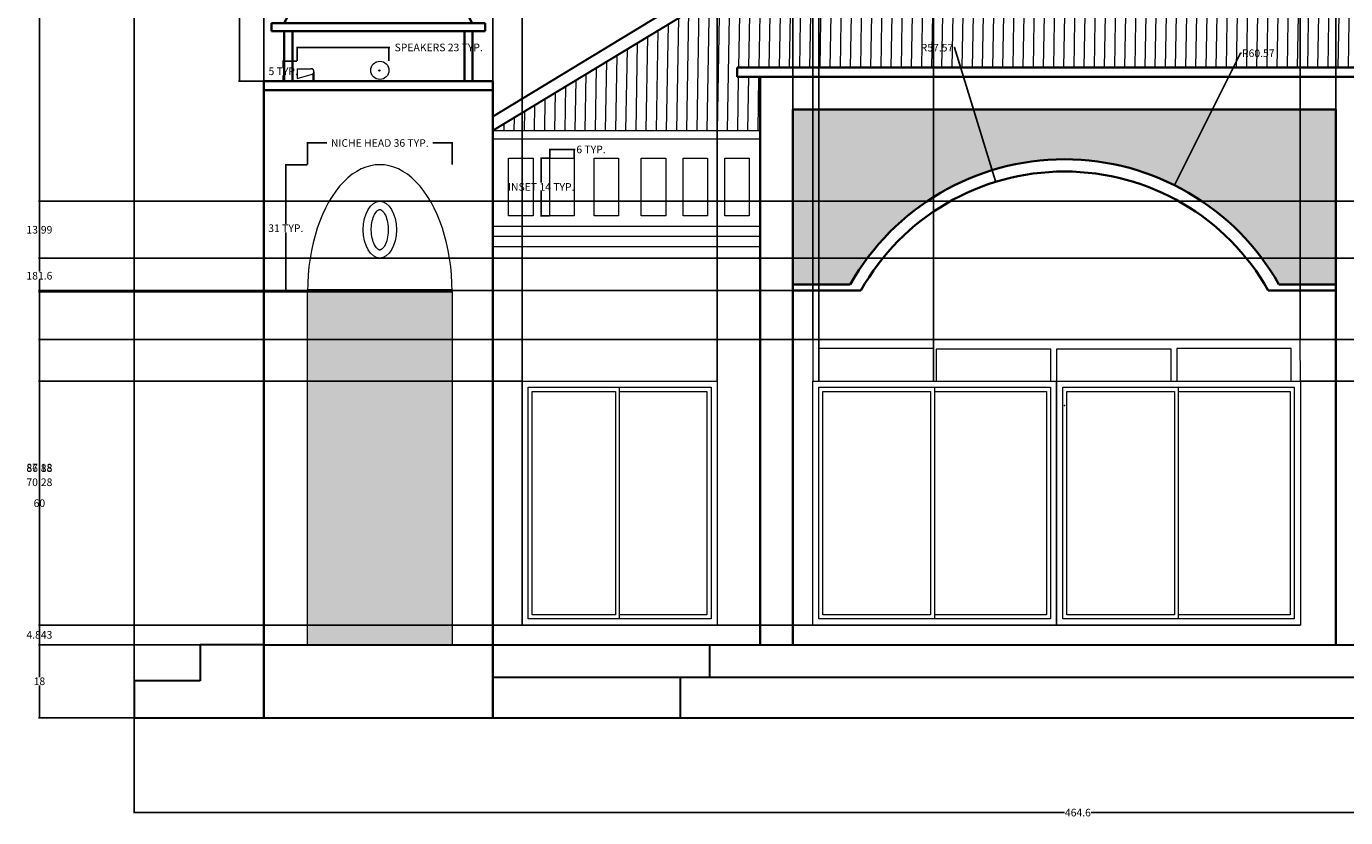
# Model space of a CAD drawing. Units: inches. Extents: x 4 to 523, y 84 to 443.
# Tile 1 of 3: x 4 to 329, y 86 to 281. Entities that reach past the tile are written whole.
import ezdxf

# ---------------------------------------------------------------- set-up
doc = ezdxf.new("R2010")
doc.units = ezdxf.units.IN
doc.header["$MEASUREMENT"] = 0
for name, color, linetype, lineweight in [('A-ANNO-DIMS', 2, 'Continuous', 18), ('A-EQPM', 8, 'Continuous', 18), ('A-FLOR-STRS', 7, 'Continuous', 30), ('A-GLAZ', 4, 'Continuous', 18), ('A-ROOF', 7, 'Continuous', 30), ('A-ROOF-DOME', 7, 'Continuous', 35), ('A-ROOF-PATT', 252, 'Continuous', 13), ('A-WALL', 7, 'Continuous', 35), ('A-WALL-PATT', 252, 'Continuous', 13), ('A-WALL-PORT', 7, 'Continuous', 35), ('A-WALL-TRIM', 3, 'Continuous', 18)]:
    doc.layers.add(name, color=color, linetype=linetype, lineweight=lineweight)
doc.styles.get("Standard").update_dxf_attribs({"font": 'arial.ttf'})
doc.dimstyles.get("Standard").update_dxf_attribs({"dimtxt": 1.875, "dimasz": 0.18, "dimexe": 0.18, "dimexo": 0.0625, "dimgap": 0.09, "dimtad": 0, "dimtih": 1, "dimtoh": 1, "dimdec": 4, "dimzin": 0, "dimdsep": 46, "dimlunit": 4, "dimtxsty": 'Standard', "dimcen": 0.09, "dimadec": 0, "dimazin": 0, "dimtfac": 1, "dimtdec": 4, "dimtofl": 0, "dimtmove": 0, "dimatfit": 3, "dimfxl": 1, "dimtolj": 1, "dimtzin": 0, "dimarcsym": 0})

# ---------------------------------------------------------------- blocks, each defined once
blk = doc.blocks.new('*U2')
for p, q in [((1.5, 1.5), (1.5, 58.5)), ((1.5, 58.5), (24, 58.5)), ((24, 1.5), (24, 58.5)), ((24, 58.5), (46.5, 58.5)), ((46.5, 58.5), (46.5, 1.5)), ((24, 1.5), (1.5, 1.5)), ((46.5, 1.5), (24, 1.5))]:
    blk.add_line(p, q)
blk.add_lwpolyline([(0, 0), (0, 60), (48, 60), (48, 0)], close=True)
for points in [[(23, 57.5), (23, 2.5), (2.5, 2.5), (2.5, 57.5), (23, 57.5)], [(24, 57.5), (45.5, 57.5), (45.5, 2.5), (24, 2.5)]]:
    blk.add_lwpolyline(points)
blk = doc.blocks.new('*U3')
for p, q in [((1.5, 1.5), (1.5, 58.5)), ((1.5, 58.5), (30, 58.5)), ((30, 1.5), (30, 58.5)), ((30, 58.5), (58.5, 58.5)), ((58.5, 58.5), (58.5, 1.5)), ((30, 1.5), (1.5, 1.5)), ((58.5, 1.5), (30, 1.5))]:
    blk.add_line(p, q)
blk.add_lwpolyline([(0, 0), (0, 60), (60, 60), (60, 0)], close=True)
for points in [[(29, 57.5), (29, 2.5), (2.5, 2.5), (2.5, 57.5), (29, 57.5)], [(30, 57.5), (57.5, 57.5), (57.5, 2.5), (30, 2.5)]]:
    blk.add_lwpolyline(points)
blk = doc.blocks.new('CUPOLA-PROFILE')
for p, q in [((52.59, 14.33), (0, 14.33)), ((0, 14.33), (0, 12.33)), ((52.59, 12.33), (52.59, 14.33)), ((0, 12.33), (52.59, 12.33)), ((3.17, 3.77), (3.17, 12.33)), ((5.17, 3.77), (5.17, 12.33)), ((47.49, 3.77), (47.49, 12.33)), ((49.49, 3.77), (49.49, 12.33)), ((3.17, 3.77), (3.17, 0)), ((5.17, 3.77), (5.17, 0)), ((47.49, 3.77), (47.49, 0)), ((49.49, 3.77), (49.49, 0))]:
    blk.add_line(p, q)
for points in [[(24.44, 39.59), (26.29, 46.64), (28.15, 39.59)], [(25.33, 38.18), (24.44, 39.59)], [(28.15, 39.59), (27.62, 38.34)], [(23.56, 34.47), (25.33, 38.18)], [(29.42, 34.47), (27.62, 38.34)], [(23.56, 34.47), (26.29, 31.2)], [(26.29, 31.2), (29.42, 34.47)], [(3.17, 14.33), (6, 19.75), (10.13, 24.22), (16.05, 28.42), (21.12, 29.8), (26.29, 31.2)], [(49.42, 14.33), (46.59, 19.75), (42.46, 24.22), (36.53, 28.42), (31.46, 29.8), (26.29, 31.2)]]:
    blk.add_lwpolyline(points)
blk = doc.blocks.new('TOWER-LOUDSPEAKERS')
for p, q in [((3.88, 1.79), (3.88, 0)), ((4.17, 2.36), (4.17, 0))]:
    blk.add_line(p, q)
for points in [[(0, 3.08), (0.04, 0.72), (3.47, 1.65)], [(0, 3.08), (3.47, 3.08)]]:
    blk.add_lwpolyline(points)
for centre, radius in [((20.39, 2.69), 2.24), ((20.27, 2.65), 0.127)]:
    blk.add_circle(centre, radius)
blk.add_arc((3.46, 2.36), 0.712, 271.2716, 91.2716)
blk = doc.blocks.new('TOWER-SHAFT')
for p, q in [((0, 0), (0, 156.67)), ((0, 156.67), (56.33, 156.67)), ((56.33, 156.67), (56.33, 0)), ((0, 154.45), (56.33, 154.45))]:
    blk.add_line(p, q)
blk = doc.blocks.new('NICHE-ARCH-MEDALLION')
blk.add_ellipse((17.8, 0), major_axis=(0, 31.26), ratio=0.569254, start_param=4.712389, end_param=7.853982)
blk.add_ellipse((17.8, 15.26), major_axis=(0, 6.99), ratio=0.584915)
blk.add_open_spline([(17.8, 20.25), (17.75, 20.25), (17.71, 20.25), (17.59, 20.21), (17.51, 20.17), (17.31, 20.03), (17.19, 19.93), (16.94, 19.66), (16.81, 19.49), (16.45, 18.9), (16.23, 18.42), (15.9, 17.3), (15.78, 16.67), (15.68, 15.37), (15.7, 14.7), (15.86, 13.43), (16, 12.82), (16.37, 11.77), (16.6, 11.33), (17.01, 10.76), (17.18, 10.58), (17.48, 10.36), (17.59, 10.31), (17.73, 10.26), (17.78, 10.26), (17.87, 10.27), (17.93, 10.28), (18.1, 10.35), (18.21, 10.42), (18.46, 10.64), (18.61, 10.8), (18.9, 11.2), (19.04, 11.44), (19.4, 12.22), (19.6, 12.82), (19.85, 14.13), (19.9, 14.84), (19.86, 16.25), (19.77, 16.94), (19.45, 18.19), (19.23, 18.74), (18.8, 19.48), (18.6, 19.73), (18.25, 20.07), (18.1, 20.16), (17.91, 20.24), (17.85, 20.25), (17.8, 20.25)], degree=3, knots=[0, 0, 0, 0, 0.190161, 0.190161, 0.380322, 0.380322, 0.570483, 0.570483, 0.760644, 0.760644, 1.099719, 1.099719, 1.438794, 1.438794, 1.77787, 1.77787, 2.116945, 2.116945, 2.45602, 2.45602, 2.714331, 2.714331, 2.972641, 2.972641, 3.185337, 3.185337, 3.398033, 3.398033, 3.610729, 3.610729, 3.823425, 3.823425, 4.03612, 4.03612, 4.39902, 4.39902, 4.76192, 4.76192, 5.124819, 5.124819, 5.487719, 5.487719, 5.764017, 5.764017, 6.040315, 6.040315, 6.283185, 6.283185, 6.283185, 6.283185])
blk = doc.blocks.new('FRIEZE-INSET')
blk.add_lwpolyline([(0, 14.2), (6.01, 14.2), (6.01, 0), (0, 0)], close=True)
blk = doc.blocks.new('*D12')
at = {"layer": 'A-ANNO-DIMS', "color": 0, "lineweight": -2, "transparency": 16777216}
for p, q in [((64.65, 313.78), (56.65, 313.78)), ((56.83, 313.6), (56.83, 291.48)), ((56.83, 267.31), (56.83, 289.43)), ((64.65, 267.13), (56.65, 267.13))]:
    blk.add_line(p, q, dxfattribs=at)
at = {"layer": 'A-ANNO-DIMS', "color": 0, "transparency": 16777216}
for points in [[(56.8, 313.6), (56.86, 313.6), (56.83, 313.78)], [(56.8, 267.31), (56.86, 267.31), (56.83, 267.13)]]:
    blk.add_solid(points, dxfattribs=at)
at = {"layer": 'Defpoints', "color": 0, "transparency": 16777216}
for p in [(56.83, 313.78), (64.71, 313.78), (64.71, 267.13)]:
    blk.add_point(p, dxfattribs=at)
at = {"layer": 'A-ANNO-DIMS', "color": 0, "transparency": 16777216, "insert": (56.83, 290.45), "char_height": 1.875, "attachment_point": 5}
blk.add_mtext('\\A1;47 TYP.', dxfattribs=at)
blk = doc.blocks.new('*D13')
at = {"layer": 'A-ANNO-DIMS', "color": 0, "lineweight": -2, "transparency": 16777216}
for p, q in [((71.01, 272.12), (71.01, 275.63)), ((71.19, 275.45), (93.46, 275.45)), ((93.64, 272.12), (93.64, 275.63)), ((93.64, 275.45), (93.82, 275.45))]:
    blk.add_line(p, q, dxfattribs=at)
at = {"layer": 'A-ANNO-DIMS', "color": 0, "transparency": 16777216}
for points in [[(71.19, 275.48), (71.19, 275.42), (71.01, 275.45)], [(93.46, 275.48), (93.46, 275.42), (93.64, 275.45)]]:
    blk.add_solid(points, dxfattribs=at)
at = {"layer": 'Defpoints', "color": 0, "transparency": 16777216}
for p in [(93.64, 275.45), (71.01, 272.06), (93.64, 272.06)]:
    blk.add_point(p, dxfattribs=at)
at = {"layer": 'A-ANNO-DIMS', "color": 0, "transparency": 16777216, "insert": (105.89, 275.45), "char_height": 1.875, "attachment_point": 5}
blk.add_mtext('\\A1;SPEAKERS 23 TYP.', dxfattribs=at)
blk = doc.blocks.new('*D14')
at = {"layer": 'A-ANNO-DIMS', "color": 0, "lineweight": -2, "transparency": 16777216}
for p, q in [((70.95, 272.06), (67.43, 272.06)), ((67.61, 271.88), (67.61, 270.64)), ((70.95, 267.13), (67.43, 267.13)), ((67.61, 267.31), (67.61, 268.55))]:
    blk.add_line(p, q, dxfattribs=at)
at = {"layer": 'A-ANNO-DIMS', "color": 0, "transparency": 16777216}
for points in [[(67.58, 271.88), (67.64, 271.88), (67.61, 272.06)], [(67.58, 267.31), (67.64, 267.31), (67.61, 267.13)]]:
    blk.add_solid(points, dxfattribs=at)
at = {"layer": 'Defpoints', "color": 0, "transparency": 16777216}
for p in [(67.61, 272.06), (71.01, 272.06), (71.01, 267.13)]:
    blk.add_point(p, dxfattribs=at)
at = {"layer": 'A-ANNO-DIMS', "color": 0, "transparency": 16777216, "insert": (67.61, 269.59), "char_height": 1.875, "attachment_point": 5}
blk.add_mtext('\\A1;5 TYP.', dxfattribs=at)
blk = doc.blocks.new('*D15')
at = {"layer": 'A-ANNO-DIMS', "color": 0, "lineweight": -2, "transparency": 16777216}
for p, q in [((73.6, 246.66), (73.6, 252.12)), ((73.78, 251.94), (78.34, 251.94)), ((109.01, 251.94), (104.44, 251.94)), ((109.19, 246.66), (109.19, 252.12))]:
    blk.add_line(p, q, dxfattribs=at)
at = {"layer": 'A-ANNO-DIMS', "color": 0, "transparency": 16777216}
for points in [[(73.78, 251.97), (73.78, 251.91), (73.6, 251.94)], [(109.01, 251.97), (109.01, 251.91), (109.19, 251.94)]]:
    blk.add_solid(points, dxfattribs=at)
at = {"layer": 'Defpoints', "color": 0, "transparency": 16777216}
for p in [(109.19, 251.94), (73.6, 246.6), (109.19, 246.6)]:
    blk.add_point(p, dxfattribs=at)
at = {"layer": 'A-ANNO-DIMS', "color": 0, "transparency": 16777216, "insert": (91.39, 251.94), "char_height": 1.875, "attachment_point": 5}
blk.add_mtext('\\A1;NICHE HEAD 36 TYP.', dxfattribs=at)
blk = doc.blocks.new('*D16')
at = {"layer": 'A-ANNO-DIMS', "color": 0, "lineweight": -2, "transparency": 16777216}
for p, q in [((73.53, 246.6), (68.08, 246.6)), ((68.26, 246.42), (68.26, 232.02)), ((68.26, 215.52), (68.26, 229.92)), ((73.53, 215.34), (68.08, 215.34))]:
    blk.add_line(p, q, dxfattribs=at)
at = {"layer": 'A-ANNO-DIMS', "color": 0, "transparency": 16777216}
for points in [[(68.23, 246.42), (68.29, 246.42), (68.26, 246.6)], [(68.23, 215.52), (68.29, 215.52), (68.26, 215.34)]]:
    blk.add_solid(points, dxfattribs=at)
at = {"layer": 'Defpoints', "color": 0, "transparency": 16777216}
for p in [(68.26, 246.6), (73.6, 246.6), (73.6, 215.34)]:
    blk.add_point(p, dxfattribs=at)
at = {"layer": 'A-ANNO-DIMS', "color": 0, "transparency": 16777216, "insert": (68.26, 230.97), "char_height": 1.875, "attachment_point": 5}
blk.add_mtext('\\A1;31 TYP.', dxfattribs=at)
blk = doc.blocks.new('*D17')
at = {"layer": 'A-ANNO-DIMS', "color": 0, "lineweight": -2, "transparency": 16777216}
for p, q in [((133.19, 248.22), (130.94, 248.22)), ((131.12, 248.04), (131.12, 242.18)), ((131.12, 234.2), (131.12, 240.06)), ((133.19, 234.02), (130.94, 234.02))]:
    blk.add_line(p, q, dxfattribs=at)
at = {"layer": 'A-ANNO-DIMS', "color": 0, "transparency": 16777216}
for points in [[(131.09, 248.04), (131.15, 248.04), (131.12, 248.22)], [(131.09, 234.2), (131.15, 234.2), (131.12, 234.02)]]:
    blk.add_solid(points, dxfattribs=at)
at = {"layer": 'Defpoints', "color": 0, "transparency": 16777216}
for p in [(131.12, 248.22), (133.25, 248.22), (133.25, 234.02)]:
    blk.add_point(p, dxfattribs=at)
at = {"layer": 'A-ANNO-DIMS', "color": 0, "transparency": 16777216, "insert": (131.12, 241.12), "char_height": 1.875, "attachment_point": 5}
blk.add_mtext('\\A1;INSET 14 TYP.', dxfattribs=at)
blk = doc.blocks.new('*D18')
at = {"layer": 'A-ANNO-DIMS', "color": 0, "lineweight": -2, "transparency": 16777216}
for p, q in [((133.25, 248.28), (133.25, 250.53)), ((133.43, 250.35), (139.08, 250.35)), ((139.26, 248.28), (139.26, 250.53)), ((139.26, 250.35), (139.44, 250.35))]:
    blk.add_line(p, q, dxfattribs=at)
at = {"layer": 'A-ANNO-DIMS', "color": 0, "transparency": 16777216}
for points in [[(133.43, 250.38), (133.43, 250.32), (133.25, 250.35)], [(139.08, 250.38), (139.08, 250.32), (139.26, 250.35)]]:
    blk.add_solid(points, dxfattribs=at)
at = {"layer": 'Defpoints', "color": 0, "transparency": 16777216}
for p in [(139.26, 250.35), (133.25, 248.22), (139.26, 248.22)]:
    blk.add_point(p, dxfattribs=at)
at = {"layer": 'A-ANNO-DIMS', "color": 0, "transparency": 16777216, "insert": (143.37, 250.35), "char_height": 1.875, "attachment_point": 5}
blk.add_mtext('\\A1;6 TYP.', dxfattribs=at)
blk = doc.blocks.new('*D19')
at = {"layer": 'A-ANNO-DIMS', "color": 0, "lineweight": -2, "transparency": 16777216}
for p, q in [((30.92, 110.4), (30.92, 86.96)), ((495.5, 110.4), (495.5, 86.96)), ((31.1, 87.14), (259.92, 87.14)), ((495.32, 87.14), (266.5, 87.14))]:
    blk.add_line(p, q, dxfattribs=at)
at = {"layer": 'A-ANNO-DIMS', "color": 0, "transparency": 16777216}
for points in [[(31.1, 87.17), (31.1, 87.11), (30.92, 87.14)], [(495.32, 87.17), (495.32, 87.11), (495.5, 87.14)]]:
    blk.add_solid(points, dxfattribs=at)
at = {"layer": 'Defpoints', "color": 0, "transparency": 16777216}
for p in [(30.92, 110.46), (495.5, 110.46), (495.5, 87.14)]:
    blk.add_point(p, dxfattribs=at)
at = {"layer": 'A-ANNO-DIMS', "color": 0, "transparency": 16777216, "insert": (263.21, 87.14), "char_height": 1.875, "attachment_point": 5}
blk.add_mtext('\\A1;464.6', dxfattribs=at)
blk = doc.blocks.new('*D20')
at = {"layer": 'A-ANNO-DIMS', "color": 0, "lineweight": -2, "transparency": 16777216}
for p, q in [((259.93, 418.56), (519, 418.56)), ((518.82, 418.38), (518.82, 265.56)), ((518.82, 110.64), (518.82, 263.46)), ((495.56, 110.46), (519, 110.46))]:
    blk.add_line(p, q, dxfattribs=at)
at = {"layer": 'A-ANNO-DIMS', "color": 0, "transparency": 16777216}
for points in [[(518.79, 418.38), (518.85, 418.38), (518.82, 418.56)], [(518.79, 110.64), (518.85, 110.64), (518.82, 110.46)]]:
    blk.add_solid(points, dxfattribs=at)
at = {"layer": 'Defpoints', "color": 0, "transparency": 16777216}
for p in [(259.87, 418.56), (518.82, 418.56), (495.5, 110.46)]:
    blk.add_point(p, dxfattribs=at)
at = {"layer": 'A-ANNO-DIMS', "color": 0, "transparency": 16777216, "insert": (518.82, 264.51), "char_height": 1.875, "attachment_point": 5}
blk.add_mtext('\\A1;308.1', dxfattribs=at)
blk = doc.blocks.new('*D21')
at = {"layer": 'A-ANNO-DIMS', "color": 0, "lineweight": -2, "transparency": 16777216}
for p, q in [((30.92, 119.64), (30.92, 442.06)), ((31.1, 441.88), (43.64, 441.88)), ((62.69, 441.88), (50.16, 441.88)), ((62.87, 128.52), (62.87, 442.06))]:
    blk.add_line(p, q, dxfattribs=at)
at = {"layer": 'A-ANNO-DIMS', "color": 0, "transparency": 16777216}
for points in [[(31.1, 441.91), (31.1, 441.85), (30.92, 441.88)], [(62.69, 441.91), (62.69, 441.85), (62.87, 441.88)]]:
    blk.add_solid(points, dxfattribs=at)
at = {"layer": 'Defpoints', "color": 0, "transparency": 16777216}
for p in [(62.87, 441.88), (62.87, 128.46), (30.92, 119.58)]:
    blk.add_point(p, dxfattribs=at)
at = {"layer": 'A-ANNO-DIMS', "color": 0, "transparency": 16777216, "insert": (46.9, 441.88), "char_height": 1.875, "attachment_point": 5}
blk.add_mtext('\\A1;31.95', dxfattribs=at)
blk = doc.blocks.new('*D23')
at = {"layer": 'A-ANNO-DIMS', "color": 0, "lineweight": -2, "transparency": 16777216}
for p, q in [((47.09, 128.46), (7.42, 128.46)), ((7.6, 128.28), (7.6, 120.51)), ((7.6, 110.64), (7.6, 118.41)), ((30.86, 110.46), (7.42, 110.46))]:
    blk.add_line(p, q, dxfattribs=at)
at = {"layer": 'A-ANNO-DIMS', "color": 0, "transparency": 16777216}
for points in [[(7.57, 128.28), (7.63, 128.28), (7.6, 128.46)], [(7.57, 110.64), (7.63, 110.64), (7.6, 110.46)]]:
    blk.add_solid(points, dxfattribs=at)
at = {"layer": 'Defpoints', "color": 0, "transparency": 16777216}
for p in [(7.6, 128.46), (47.15, 128.46), (30.92, 110.46)]:
    blk.add_point(p, dxfattribs=at)
at = {"layer": 'A-ANNO-DIMS', "color": 0, "transparency": 16777216, "insert": (7.6, 119.46), "char_height": 1.875, "attachment_point": 5}
blk.add_mtext('\\A1;18', dxfattribs=at)
blk = doc.blocks.new('*D24')
at = {"layer": 'A-ANNO-DIMS', "color": 0, "lineweight": -2, "transparency": 16777216}
for p, q in [((168.55, 310.07), (7.42, 310.07)), ((7.6, 309.89), (7.6, 220.31)), ((7.6, 128.64), (7.6, 218.22)), ((47.09, 128.46), (7.42, 128.46))]:
    blk.add_line(p, q, dxfattribs=at)
at = {"layer": 'A-ANNO-DIMS', "color": 0, "transparency": 16777216}
for points in [[(7.57, 309.89), (7.63, 309.89), (7.6, 310.07)], [(7.57, 128.64), (7.63, 128.64), (7.6, 128.46)]]:
    blk.add_solid(points, dxfattribs=at)
at = {"layer": 'Defpoints', "color": 0, "transparency": 16777216}
for p in [(7.6, 310.07), (168.61, 310.07), (47.15, 128.46)]:
    blk.add_point(p, dxfattribs=at)
at = {"layer": 'A-ANNO-DIMS', "color": 0, "transparency": 16777216, "insert": (7.6, 219.27), "char_height": 1.875, "attachment_point": 5}
blk.add_mtext('\\A1;181.6', dxfattribs=at)
blk = doc.blocks.new('*D28')
at = {"layer": 'A-ANNO-DIMS', "color": 0, "lineweight": -2, "transparency": 16777216}
for p, q in [((193.01, 215.71), (193.01, 442.06)), ((193.19, 441.88), (255.99, 441.88)), ((326.55, 441.88), (263.75, 441.88)), ((326.73, 215.71), (326.73, 442.06))]:
    blk.add_line(p, q, dxfattribs=at)
at = {"layer": 'A-ANNO-DIMS', "color": 0, "transparency": 16777216}
for points in [[(193.19, 441.91), (193.19, 441.85), (193.01, 441.88)], [(326.55, 441.91), (326.55, 441.85), (326.73, 441.88)]]:
    blk.add_solid(points, dxfattribs=at)
at = {"layer": 'Defpoints', "color": 0, "transparency": 16777216}
for p in [(326.73, 441.88), (193.01, 215.64), (326.73, 215.64)]:
    blk.add_point(p, dxfattribs=at)
at = {"layer": 'A-ANNO-DIMS', "color": 0, "transparency": 16777216, "insert": (259.87, 441.88), "char_height": 1.875, "attachment_point": 5}
blk.add_mtext('\\A1;133.72', dxfattribs=at)
blk = doc.blocks.new('*D29')
at = {"layer": 'A-ANNO-DIMS', "color": 0, "lineweight": -2, "transparency": 16777216}
for p, q in [((192.95, 215.64), (7.42, 215.64)), ((7.6, 215.46), (7.6, 173.1)), ((7.6, 128.64), (7.6, 171)), ((192.95, 128.46), (7.42, 128.46))]:
    blk.add_line(p, q, dxfattribs=at)
at = {"layer": 'A-ANNO-DIMS', "color": 0, "transparency": 16777216}
for points in [[(7.57, 215.46), (7.63, 215.46), (7.6, 215.64)], [(7.57, 128.64), (7.63, 128.64), (7.6, 128.46)]]:
    blk.add_solid(points, dxfattribs=at)
at = {"layer": 'Defpoints', "color": 0, "transparency": 16777216}
for p in [(7.6, 215.64), (193.01, 215.64), (193.01, 128.46)]:
    blk.add_point(p, dxfattribs=at)
at = {"layer": 'A-ANNO-DIMS', "color": 0, "transparency": 16777216, "insert": (7.6, 172.05), "char_height": 1.875, "attachment_point": 5}
blk.add_mtext('\\A1;87.18', dxfattribs=at)
blk = doc.blocks.new('*D30')
at = {"layer": 'A-ANNO-DIMS', "color": 0, "lineweight": -2, "transparency": 16777216}
for p, q in [((126.41, 193.37), (126.41, 442.06)), ((126.59, 441.88), (148.94, 441.88)), ((174.23, 441.88), (151.88, 441.88)), ((174.41, 193.37), (174.41, 442.06))]:
    blk.add_line(p, q, dxfattribs=at)
at = {"layer": 'A-ANNO-DIMS', "color": 0, "transparency": 16777216}
for points in [[(126.59, 441.91), (126.59, 441.85), (126.41, 441.88)], [(174.23, 441.91), (174.23, 441.85), (174.41, 441.88)]]:
    blk.add_solid(points, dxfattribs=at)
at = {"layer": 'Defpoints', "color": 0, "transparency": 16777216}
for p in [(174.41, 441.88), (126.41, 193.3), (174.41, 193.3)]:
    blk.add_point(p, dxfattribs=at)
at = {"layer": 'A-ANNO-DIMS', "color": 0, "transparency": 16777216, "insert": (150.41, 441.88), "char_height": 1.875, "attachment_point": 5}
blk.add_mtext('\\A1;48', dxfattribs=at)
blk = doc.blocks.new('*D31')
at = {"layer": 'A-ANNO-DIMS', "color": 0, "lineweight": -2, "transparency": 16777216}
for p, q in [((126.35, 193.3), (7.42, 193.3)), ((7.6, 193.12), (7.6, 164.35)), ((7.6, 133.48), (7.6, 162.26)), ((126.35, 133.3), (7.42, 133.3))]:
    blk.add_line(p, q, dxfattribs=at)
at = {"layer": 'A-ANNO-DIMS', "color": 0, "transparency": 16777216}
for points in [[(7.57, 193.12), (7.63, 193.12), (7.6, 193.3)], [(7.57, 133.48), (7.63, 133.48), (7.6, 133.3)]]:
    blk.add_solid(points, dxfattribs=at)
at = {"layer": 'Defpoints', "color": 0, "transparency": 16777216}
for p in [(7.6, 193.3), (126.41, 193.3), (126.41, 133.3)]:
    blk.add_point(p, dxfattribs=at)
at = {"layer": 'A-ANNO-DIMS', "color": 0, "transparency": 16777216, "insert": (7.6, 163.3), "char_height": 1.875, "attachment_point": 5}
blk.add_mtext('\\A1;60', dxfattribs=at)
blk = doc.blocks.new('*D32')
at = {"layer": 'A-ANNO-DIMS', "color": 0, "lineweight": -2, "transparency": 16777216}
for p, q in [((197.96, 203.64), (197.96, 442.06)), ((198.14, 441.88), (254.04, 441.88)), ((317.74, 441.88), (261.84, 441.88)), ((317.92, 203.64), (317.92, 442.06))]:
    blk.add_line(p, q, dxfattribs=at)
at = {"layer": 'A-ANNO-DIMS', "color": 0, "transparency": 16777216}
for points in [[(198.14, 441.91), (198.14, 441.85), (197.96, 441.88)], [(317.74, 441.91), (317.74, 441.85), (317.92, 441.88)]]:
    blk.add_solid(points, dxfattribs=at)
at = {"layer": 'Defpoints', "color": 0, "transparency": 16777216}
for p in [(317.92, 441.88), (197.96, 203.58), (317.92, 203.58)]:
    blk.add_point(p, dxfattribs=at)
at = {"layer": 'A-ANNO-DIMS', "color": 0, "transparency": 16777216, "insert": (257.94, 441.88), "char_height": 1.875, "attachment_point": 5}
blk.add_mtext('\\A1;119.95', dxfattribs=at)
blk = doc.blocks.new('*D33')
at = {"layer": 'A-ANNO-DIMS', "color": 0, "lineweight": -2, "transparency": 16777216}
for p, q in [((317.85, 203.58), (7.42, 203.58)), ((7.6, 203.4), (7.6, 169.49)), ((7.6, 133.48), (7.6, 167.4)), ((317.9, 133.3), (7.42, 133.3))]:
    blk.add_line(p, q, dxfattribs=at)
at = {"layer": 'A-ANNO-DIMS', "color": 0, "transparency": 16777216}
for points in [[(7.57, 203.4), (7.63, 203.4), (7.6, 203.58)], [(7.57, 133.48), (7.63, 133.48), (7.6, 133.3)]]:
    blk.add_solid(points, dxfattribs=at)
at = {"layer": 'Defpoints', "color": 0, "transparency": 16777216}
for p in [(7.6, 203.58), (317.92, 203.58), (317.96, 133.3)]:
    blk.add_point(p, dxfattribs=at)
at = {"layer": 'A-ANNO-DIMS', "color": 0, "transparency": 16777216, "insert": (7.6, 168.44), "char_height": 1.875, "attachment_point": 5}
blk.add_mtext('\\A1;70.28', dxfattribs=at)
blk = doc.blocks.new('*D34')
at = {"layer": 'A-ANNO-DIMS', "color": 0, "lineweight": -2, "transparency": 16777216}
for p, q in [((73.53, 215.34), (7.42, 215.34)), ((7.6, 215.16), (7.6, 172.95)), ((7.6, 128.64), (7.6, 170.85)), ((73.53, 128.46), (7.42, 128.46))]:
    blk.add_line(p, q, dxfattribs=at)
at = {"layer": 'A-ANNO-DIMS', "color": 0, "transparency": 16777216}
for points in [[(7.57, 215.16), (7.63, 215.16), (7.6, 215.34)], [(7.57, 128.64), (7.63, 128.64), (7.6, 128.46)]]:
    blk.add_solid(points, dxfattribs=at)
at = {"layer": 'Defpoints', "color": 0, "transparency": 16777216}
for p in [(7.6, 215.34), (73.6, 215.34), (73.6, 128.46)]:
    blk.add_point(p, dxfattribs=at)
at = {"layer": 'A-ANNO-DIMS', "color": 0, "transparency": 16777216, "insert": (7.6, 171.9), "char_height": 1.875, "attachment_point": 5}
blk.add_mtext('\\A1;86.88', dxfattribs=at)
blk = doc.blocks.new('*D35')
at = {"layer": 'A-ANNO-DIMS', "color": 0, "lineweight": -2, "transparency": 16777216}
for p, q in [((174.35, 133.3), (7.42, 133.3)), ((7.6, 133.12), (7.6, 131.93)), ((172.5, 128.46), (7.42, 128.46)), ((7.6, 128.64), (7.6, 129.83))]:
    blk.add_line(p, q, dxfattribs=at)
at = {"layer": 'A-ANNO-DIMS', "color": 0, "transparency": 16777216}
for points in [[(7.57, 133.12), (7.63, 133.12), (7.6, 133.3)], [(7.57, 128.64), (7.63, 128.64), (7.6, 128.46)]]:
    blk.add_solid(points, dxfattribs=at)
at = {"layer": 'Defpoints', "color": 0, "transparency": 16777216}
for p in [(174.41, 133.3), (7.6, 128.46), (172.56, 128.46)]:
    blk.add_point(p, dxfattribs=at)
at = {"layer": 'A-ANNO-DIMS', "color": 0, "transparency": 16777216, "insert": (7.6, 130.88), "char_height": 1.875, "attachment_point": 5}
blk.add_mtext('\\A1;4.843', dxfattribs=at)
blk = doc.blocks.new('*D36')
at = {"layer": 'A-ANNO-DIMS', "color": 0, "lineweight": -2, "transparency": 16777216}
for p, q in [((119.21, 120.55), (119.21, 442.06)), ((119.39, 441.88), (119.57, 441.88)), ((126.23, 441.88), (126.05, 441.88)), ((126.41, 133.37), (126.41, 442.06))]:
    blk.add_line(p, q, dxfattribs=at)
at = {"layer": 'A-ANNO-DIMS', "color": 0, "transparency": 16777216}
for points in [[(119.39, 441.91), (119.39, 441.85), (119.21, 441.88)], [(126.23, 441.91), (126.23, 441.85), (126.41, 441.88)]]:
    blk.add_solid(points, dxfattribs=at)
at = {"layer": 'Defpoints', "color": 0, "transparency": 16777216}
for p in [(126.41, 441.88), (126.41, 133.3), (119.21, 120.48)]:
    blk.add_point(p, dxfattribs=at)
at = {"layer": 'A-ANNO-DIMS', "color": 0, "transparency": 16777216, "insert": (122.81, 441.88), "char_height": 1.875, "attachment_point": 5}
blk.add_mtext('\\A1;7.202', dxfattribs=at)
blk = doc.blocks.new('*D37')
at = {"layer": 'A-ANNO-DIMS', "color": 0, "lineweight": -2, "transparency": 16777216}
for p, q in [((317.98, 203.58), (519, 203.58)), ((518.82, 203.4), (518.82, 199.49)), ((518.82, 193.48), (518.82, 197.4)), ((318.02, 193.3), (519, 193.3))]:
    blk.add_line(p, q, dxfattribs=at)
at = {"layer": 'A-ANNO-DIMS', "color": 0, "transparency": 16777216}
for points in [[(518.79, 203.4), (518.85, 203.4), (518.82, 203.58)], [(518.79, 193.48), (518.85, 193.48), (518.82, 193.3)]]:
    blk.add_solid(points, dxfattribs=at)
at = {"layer": 'Defpoints', "color": 0, "transparency": 16777216}
for p in [(317.92, 203.58), (317.96, 193.3), (518.82, 193.3)]:
    blk.add_point(p, dxfattribs=at)
at = {"layer": 'A-ANNO-DIMS', "color": 0, "transparency": 16777216, "insert": (518.82, 198.44), "char_height": 1.875, "attachment_point": 5}
blk.add_mtext('\\A1;10.278', dxfattribs=at)
blk = doc.blocks.new('*D39')
at = {"layer": 'A-ANNO-DIMS', "color": 0, "lineweight": -2, "transparency": 16777216}
for p, q in [((199.46, 193.37), (199.46, 442.06)), ((199.64, 441.88), (210.28, 441.88)), ((227.46, 441.88), (216.82, 441.88)), ((227.64, 193.37), (227.64, 442.06))]:
    blk.add_line(p, q, dxfattribs=at)
at = {"layer": 'A-ANNO-DIMS', "color": 0, "transparency": 16777216}
for points in [[(199.64, 441.91), (199.64, 441.85), (199.46, 441.88)], [(227.46, 441.91), (227.46, 441.85), (227.64, 441.88)]]:
    blk.add_solid(points, dxfattribs=at)
at = {"layer": 'Defpoints', "color": 0, "transparency": 16777216}
for p in [(227.64, 441.88), (199.46, 193.3), (227.64, 193.3)]:
    blk.add_point(p, dxfattribs=at)
at = {"layer": 'A-ANNO-DIMS', "color": 0, "transparency": 16777216, "insert": (213.55, 441.88), "char_height": 1.875, "attachment_point": 5}
blk.add_mtext('\\A1;28.18', dxfattribs=at)
blk = doc.blocks.new('*D41')
at = {"layer": 'A-ANNO-DIMS', "color": 0, "lineweight": -2, "transparency": 16777216}
for p, q in [((428.29, 237.59), (7.42, 237.59)), ((7.6, 237.41), (7.6, 231.64)), ((7.6, 223.78), (7.6, 229.55)), ((428.29, 223.6), (7.42, 223.6))]:
    blk.add_line(p, q, dxfattribs=at)
at = {"layer": 'A-ANNO-DIMS', "color": 0, "transparency": 16777216}
for points in [[(7.57, 237.41), (7.63, 237.41), (7.6, 237.59)], [(7.57, 223.78), (7.63, 223.78), (7.6, 223.6)]]:
    blk.add_solid(points, dxfattribs=at)
at = {"layer": 'Defpoints', "color": 0, "transparency": 16777216}
for p in [(428.35, 237.59), (7.6, 223.6), (428.35, 223.6)]:
    blk.add_point(p, dxfattribs=at)
at = {"layer": 'A-ANNO-DIMS', "color": 0, "transparency": 16777216, "insert": (7.6, 230.59), "char_height": 1.875, "attachment_point": 5}
blk.add_mtext('\\A1;13.99', dxfattribs=at)
blk = doc.blocks.new('*D43')
at = {"layer": 'A-ANNO-DIMS', "color": 0, "lineweight": -2, "transparency": 16777216}
for p, q in [((303.27, 274.03), (287.09, 241.69)), ((303.45, 274.03), (303.27, 274.03)), ((259.83, 187.36), (260.01, 187.36)), ((259.92, 187.27), (259.92, 187.45))]:
    blk.add_line(p, q, dxfattribs=at)
at = {"layer": 'A-ANNO-DIMS', "color": 0, "transparency": 16777216}
blk.add_solid([(287.07, 241.7), (287.12, 241.68), (287.01, 241.53)], dxfattribs=at)
at = {"layer": 'Defpoints', "color": 0, "transparency": 16777216}
for p in [(287.01, 241.53), (259.92, 187.36)]:
    blk.add_point(p, dxfattribs=at)
at = {"layer": 'A-ANNO-DIMS', "color": 0, "transparency": 16777216, "insert": (307.6, 274.03), "char_height": 1.875, "attachment_point": 5}
blk.add_mtext('\\A1;R60.57', dxfattribs=at)
blk = doc.blocks.new('*D44')
at = {"layer": 'A-ANNO-DIMS', "color": 0, "lineweight": -2, "transparency": 16777216}
for p, q in [((232.67, 275.4), (232.85, 275.4)), ((232.85, 275.4), (242.95, 242.55)), ((259.83, 187.36), (260.01, 187.36)), ((259.92, 187.27), (259.92, 187.45))]:
    blk.add_line(p, q, dxfattribs=at)
at = {"layer": 'A-ANNO-DIMS', "color": 0, "transparency": 16777216}
blk.add_solid([(242.98, 242.56), (242.92, 242.55), (243.01, 242.38)], dxfattribs=at)
at = {"layer": 'Defpoints', "color": 0, "transparency": 16777216}
for p in [(243.01, 242.38), (259.92, 187.36)]:
    blk.add_point(p, dxfattribs=at)
at = {"layer": 'A-ANNO-DIMS', "color": 0, "transparency": 16777216, "insert": (228.52, 275.4), "char_height": 1.875, "attachment_point": 5}
blk.add_mtext('\\A1;R57.57', dxfattribs=at)

msp = doc.modelspace()

# ---------------------------------------------------------------- hatches: boundary and pattern name
at = {"layer": 'A-ROOF-PATT'}
h = msp.add_hatch(dxfattribs=at)
h.set_pattern_fill('ANSI31', color=256, scale=20, angle=44)
h.paths.add_polyline_path([(335.7846, 294.2465), (329.6848, 294.2465), (259.8699, 294.2465), (190.0549, 294.2465), (183.9551, 294.2465), (119.2078, 254.9874), (185.0083, 254.9874), (185.0083, 259.3969), (185.0083, 268.2159), (179.3813, 268.2159), (179.3813, 270.5155), (240.8614, 270.5155), (259.8699, 270.5155), (278.8783, 270.5155), (340.3584, 270.5155), (340.3584, 268.2159), (334.7314, 268.2159), (334.7314, 259.3969), (334.7314, 254.9874), (400.5319, 254.9874)])
at = {"layer": 'A-WALL-PATT'}
h = msp.add_hatch(dxfattribs=at)
h.set_pattern_fill('ESCHER', color=256, scale=7.5)
h.paths.add_polyline_path([(109.1877, 215.3374), (73.596, 215.3374), (73.596, 128.4611), (109.1877, 128.4611)])
h.paths.add_polyline_path([(446.1437, 215.3374), (410.5521, 215.3374), (410.5521, 128.4611), (446.1437, 128.4611)])
h.paths.add_polyline_path([(326.7314, 260.2159), (259.8699, 260.2159), (193.0083, 260.2159), (193.0083, 217.1172), (203.3352, 217.1172), (207.1721, 217.1172, -0.58399271), (312.6778, 217.1172), (316.4045, 217.1172), (326.7314, 217.1172)])

# ---------------------------------------------------------------- linework, layer by layer
at = {"layer": 'A-FLOR-STRS'}
for p, q in [((62.873, 128.4611), (47.1512, 128.4611)), ((47.1512, 128.4611), (47.1512, 119.5803)), ((62.873, 110.4611), (62.873, 128.4611)), ((62.873, 128.4611), (463.5437, 128.4611)), ((172.5636, 128.4611), (172.5636, 120.483)), ((119.2078, 120.483), (400.5319, 120.483)), ((165.3007, 120.483), (165.3007, 110.4611)), ((47.1512, 119.5803), (30.9213, 119.5803)), ((30.9213, 119.5803), (30.9213, 110.4611)), ((30.9213, 110.4611), (42.685, 110.4611)), ((42.685, 110.4611), (229.6366, 110.4611)), ((229.6366, 110.4611), (465.7812, 110.4611))]:
    msp.add_line(p, q, dxfattribs=at)
at = {"layer": 'A-GLAZ'}
for points in [[(197.9616, 193.3038), (317.9616, 193.3038), (317.9162, 203.5817), (197.9616, 203.5817)], [(199.4616, 193.3038), (227.6434, 193.3038), (227.6434, 201.3359), (199.4616, 201.3359)], [(287.5556, 193.3038), (315.7375, 193.3038), (315.7375, 201.3359), (287.5556, 201.3359)], [(228.3531, 193.3038), (256.535, 193.3038), (256.535, 201.1802), (228.3531, 201.1802)], [(257.9544, 193.3038), (286.1363, 193.3038), (286.1363, 201.1802), (257.9544, 201.1802)]]:
    msp.add_lwpolyline(points, close=True, dxfattribs=at)
at = {"layer": 'A-ROOF'}
for p, q in [((119.2078, 254.9874), (183.9551, 294.2465)), ((119.2078, 258.4958), (178.169, 294.2465))]:
    msp.add_line(p, q, dxfattribs=at)
at = {"layer": 'A-WALL-PORT'}
for p, q in [((179.3813, 270.5155), (240.8614, 270.5155)), ((179.3813, 270.5155), (179.3813, 268.2159)), ((240.8614, 270.5155), (259.8699, 270.5155)), ((278.8783, 270.5155), (259.8699, 270.5155)), ((340.3584, 270.5155), (278.8783, 270.5155)), ((185.0083, 268.2159), (179.3813, 268.2159)), ((185.0083, 259.3969), (185.0083, 268.2159)), ((185.0083, 268.2159), (259.8699, 268.2159)), ((334.7314, 268.2159), (259.8699, 268.2159)), ((193.0083, 217.1172), (193.0083, 260.2159)), ((193.0083, 260.2159), (259.8699, 260.2159)), ((326.7314, 260.2159), (259.8699, 260.2159)), ((326.7314, 217.1172), (326.7314, 260.2159)), ((185.0083, 259.3969), (185.0083, 254.9874)), ((185.0083, 254.9874), (185.0083, 128.4611)), ((193.0083, 217.1172), (193.0083, 128.4611)), ((193.0083, 217.1172), (203.3352, 217.1172)), ((209.785, 215.6431), (193.0083, 215.6431)), ((203.3352, 217.1172), (207.1721, 217.1172)), ((310.0649, 215.6431), (326.7314, 215.6431)), ((316.4045, 217.1172), (312.6778, 217.1172)), ((326.7314, 217.1172), (316.4045, 217.1172)), ((326.7314, 217.1172), (326.7314, 128.4611))]:
    msp.add_line(p, q, dxfattribs=at)
for radius in [60.5693, 57.5693]:
    msp.add_arc((259.925, 187.3552), radius, 29.430766, 150.569234, dxfattribs=at)
at = {"layer": 'A-WALL-TRIM'}
for p, q in [((119.2078, 254.9874), (185.0083, 254.9874)), ((119.2078, 252.9874), (185.0083, 252.9874)), ((119.2078, 231.4916), (185.0083, 231.4916)), ((119.2078, 228.9916), (185.0083, 228.9916)), ((119.2078, 226.4916), (185.0083, 226.4916)), ((73.5992, 215.9247), (109.1849, 215.8835))]:
    msp.add_line(p, q, dxfattribs=at)
msp.add_lwpolyline([(73.596, 215.3374), (109.1877, 215.3374), (109.1877, 128.4611), (73.596, 128.4611)], close=True, dxfattribs=at)

# ---------------------------------------------------------------- block references
at = {"layer": 'A-EQPM'}
msp.add_blockref('TOWER-LOUDSPEAKERS', (71.008, 267.131), dxfattribs=at)
at = {"layer": 'A-GLAZ'}
for name, p in [('*U2', (126.4097, 133.3038)), ('*U3', (197.9616, 133.3038)), ('*U3', (257.9616, 133.3038))]:
    msp.add_blockref(name, p, dxfattribs=at)
at = {"layer": 'A-ROOF-DOME'}
msp.add_blockref('CUPOLA-PROFILE', (64.714, 267.131), dxfattribs=at)
at = {"layer": 'A-WALL'}
msp.add_blockref('TOWER-SHAFT', (62.873, 110.461), dxfattribs=at)
at = {"layer": 'A-WALL-TRIM'}
for name, p in [('FRIEZE-INSET', (123.1, 234.017)), ('FRIEZE-INSET', (133.2526, 234.017)), ('FRIEZE-INSET', (144.1361, 234.017)), ('FRIEZE-INSET', (155.7507, 234.017)), ('FRIEZE-INSET', (166.0657, 234.017)), ('FRIEZE-INSET', (176.2995, 234.017)), ('NICHE-ARCH-MEDALLION', (73.596, 215.337))]:
    msp.add_blockref(name, p, dxfattribs=at)

# ---------------------------------------------------------------- dimensions: what is measured, and where the dimension line sits
at = {"layer": 'A-ANNO-DIMS'}
for base, p1, p2, override, picture, middle in [((62.873, 441.8826), (30.9213, 119.5803), (62.873, 128.4611), {"dimdec": 2, "dimlfac": 1, "dimrnd": 0, "dimzin": 0, "dimdsep": 46, "dimlunit": 2}, '*D21', (46.8972, 441.8826)), ((126.4097, 441.8826), (119.2078, 120.483), (126.4097, 133.3038), {"dimdec": 3, "dimlfac": 1, "dimrnd": 0, "dimzin": 0, "dimdsep": 46, "dimlunit": 2}, '*D36', (122.8087, 441.8826)), ((174.4097, 441.8826), (126.4097, 193.3038), (174.4097, 193.3038), {"dimdec": 0, "dimlfac": 1, "dimrnd": 0, "dimzin": 0, "dimdsep": 46, "dimlunit": 2}, '*D30', (150.4097, 441.8826)), ((326.7314, 441.8826), (193.0083, 215.6431), (326.7314, 215.6431), {"dimdec": 2, "dimlfac": 1, "dimrnd": 0, "dimzin": 0, "dimdsep": 46, "dimlunit": 2}, '*D28', (259.8699, 441.8826)), ((317.9162, 441.8826), (197.9616, 203.5817), (317.9162, 203.5817), {"dimdec": 2, "dimlfac": 1, "dimrnd": 0, "dimzin": 0, "dimdsep": 46, "dimlunit": 2}, '*D32', (257.9389, 441.8826)), ((227.6434, 441.8826), (199.4616, 193.3038), (227.6434, 193.3038), {"dimdec": 2, "dimlfac": 1, "dimrnd": 0, "dimzin": 0, "dimdsep": 46, "dimlunit": 2}, '*D39', (213.5525, 441.8826)), ((495.4954, 87.1361), (30.9213, 110.4611), (495.4954, 110.4611), {"dimdec": 1, "dimlfac": 1, "dimrnd": 0, "dimzin": 0, "dimdsep": 46, "dimlunit": 2}, '*D19', (263.2083, 87.1361))]:
    dim = msp.add_linear_dim(base=base, p1=p1, p2=p2, dimstyle='Standard', override=override, dxfattribs=at)
    dim.commit()
    dim.dimension.update_dxf_attribs({"geometry": picture, "text_midpoint": middle})
for base, p1, p2, override, picture, middle in [((518.8204, 418.5576), (495.4954, 110.4611), (259.8702, 418.5576), {"dimdec": 1, "dimlfac": 1, "dimrnd": 0, "dimzin": 0, "dimdsep": 46, "dimlunit": 2}, '*D20', (518.8204, 264.5094)), ((7.5963, 310.0699), (47.1512, 128.4611), (168.6117, 310.0699), {"dimdec": 1, "dimlfac": 1, "dimrnd": 0, "dimzin": 0, "dimdsep": 46, "dimlunit": 2}, '*D24', (7.5963, 219.2655)), ((7.5963, 223.6005), (428.3479, 237.5894), (428.3479, 223.6005), {"dimdec": 2, "dimlfac": 1, "dimrnd": 0, "dimzin": 0, "dimdsep": 46, "dimlunit": 2}, '*D41', (7.5963, 230.595)), ((7.5963, 215.6431), (193.0083, 128.4611), (193.0083, 215.6431), {"dimdec": 2, "dimlfac": 1, "dimrnd": 0, "dimzin": 0, "dimdsep": 46, "dimlunit": 2}, '*D29', (7.5963, 172.0521)), ((7.5963, 215.3374), (73.596, 128.4611), (73.596, 215.3374), {"dimdec": 2, "dimlfac": 1, "dimrnd": 0, "dimzin": 0, "dimdsep": 46, "dimlunit": 2}, '*D34', (7.5963, 171.8992)), ((7.5963, 203.5817), (317.9616, 133.3038), (317.9162, 203.5817), {"dimdec": 2, "dimlfac": 1, "dimrnd": 0, "dimzin": 0, "dimdsep": 46, "dimlunit": 2}, '*D33', (7.5963, 168.4427)), ((518.8204, 193.3038), (317.9162, 203.5817), (317.9616, 193.3038), {"dimdec": 3, "dimlfac": 1, "dimrnd": 0, "dimzin": 0, "dimdsep": 46, "dimlunit": 2}, '*D37', (518.8204, 198.4427)), ((7.5963, 193.3038), (126.4097, 133.3038), (126.4097, 193.3038), {"dimdec": 0, "dimlfac": 1, "dimrnd": 0, "dimzin": 0, "dimdsep": 46, "dimlunit": 2}, '*D31', (7.5963, 163.3038)), ((7.5963, 128.4611), (174.4097, 133.3038), (172.5636, 128.4611), {"dimdec": 3, "dimlfac": 1, "dimrnd": 0, "dimzin": 0, "dimdsep": 46, "dimlunit": 2}, '*D35', (7.5963, 130.8824)), ((7.5963, 128.4611), (30.9213, 110.4611), (47.1512, 128.4611), {"dimdec": 0, "dimlfac": 1, "dimrnd": 0, "dimzin": 0, "dimdsep": 46, "dimlunit": 2}, '*D23', (7.5963, 119.4611))]:
    dim = msp.add_linear_dim(base=base, p1=p1, p2=p2, angle=90, dimstyle='Standard', override=override, dxfattribs=at)
    dim.commit()
    dim.dimension.update_dxf_attribs({"geometry": picture, "text_midpoint": middle})
for base, p1, p2, text, picture, middle in [((56.8261, 313.7758), (64.7144, 267.1306), (64.7144, 313.7758), '<> TYP.', '*D12', (56.8261, 290.4532)), ((67.6132, 272.0593), (71.0076, 267.1306), (71.0076, 272.0593), '<> TYP.', '*D14', (67.6132, 269.5949)), ((131.1223, 248.2188), (133.2526, 234.0166), (133.2526, 248.2188), 'INSET <> TYP.', '*D17', (131.1223, 241.1177)), ((68.2573, 246.599), (73.596, 215.3374), (73.596, 246.599), '<> TYP.', '*D16', (68.2573, 230.9682))]:
    dim = msp.add_linear_dim(base=base, p1=p1, p2=p2, angle=90, text=text, dimstyle='Standard', override={"dimdec": 0, "dimlfac": 1, "dimrnd": 0, "dimzin": 0, "dimdsep": 46, "dimlunit": 2}, dxfattribs=at)
    dim.commit()
    dim.dimension.update_dxf_attribs({"geometry": picture, "text_midpoint": middle})
for base, p1, p2, text, picture, middle in [((93.6368, 275.4537), (71.0076, 272.0593), (93.6368, 272.0593), 'SPEAKERS <> TYP.', '*D13', (105.8903, 275.4537)), ((109.1877, 251.9377), (73.596, 246.599), (109.1877, 246.599), 'NICHE HEAD <> TYP.', '*D15', (91.3918, 251.9377)), ((139.2629, 250.3491), (133.2526, 248.2188), (139.2629, 248.2188), '<> TYP.', '*D18', (143.3731, 250.3491))]:
    dim = msp.add_linear_dim(base=base, p1=p1, p2=p2, text=text, dimstyle='Standard', override={"dimdec": 0, "dimlfac": 1, "dimrnd": 0, "dimzin": 0, "dimdsep": 46, "dimlunit": 2}, dxfattribs=at)
    dim.commit()
    dim.dimension.update_dxf_attribs({"geometry": picture, "text_midpoint": middle})
for mpoint, picture, middle in [((243.0055, 242.3821), '*D44', (228.523, 275.3982)), ((287.0145, 241.529), '*D43', (307.599, 274.0332))]:
    dim = msp.add_radius_dim(center=(259.925, 187.3552), mpoint=mpoint, dimstyle='Standard', override={"dimdec": 2, "dimlfac": 1, "dimrnd": 0, "dimzin": 0, "dimdsep": 46, "dimlunit": 2}, dxfattribs=at)
    dim.commit()
    dim.dimension.update_dxf_attribs({"geometry": picture, "text_midpoint": middle, "dimtype": 164})

doc.saveas('drawing.dxf')
